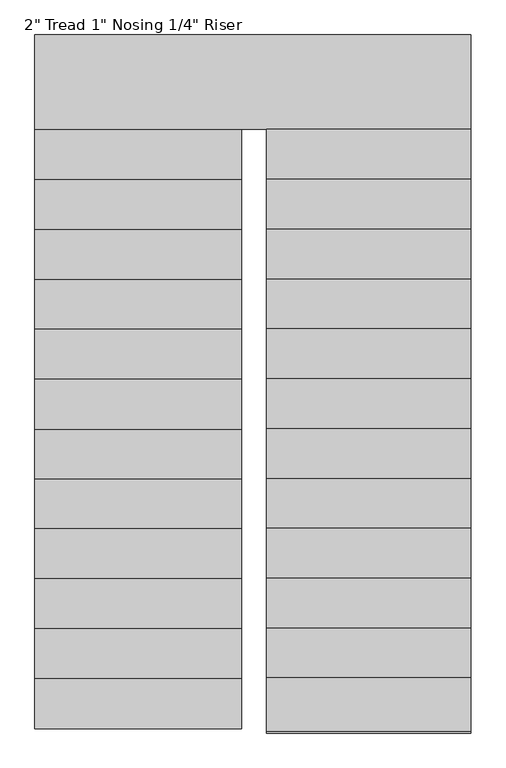
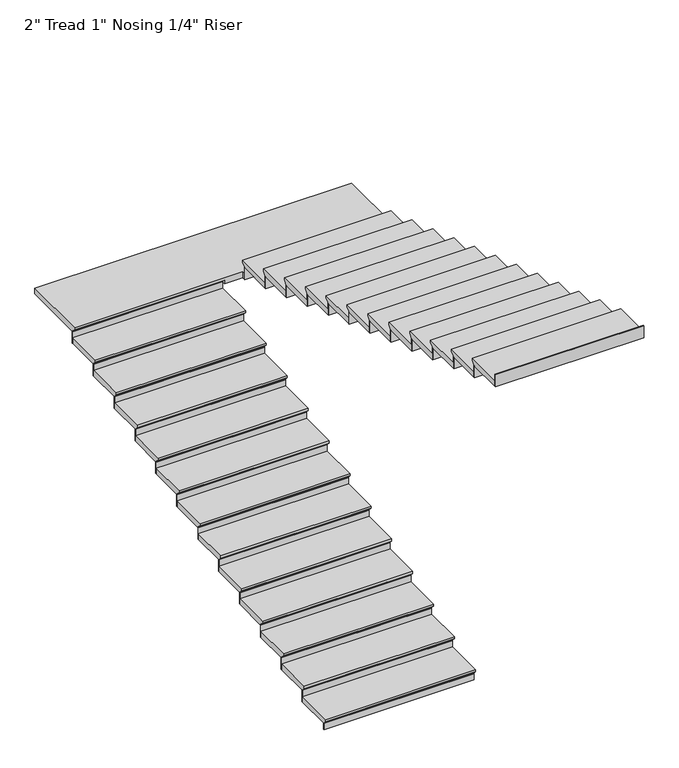
"""IFC4 building model written with IfcOpenShell, lengths in millimetres: stair flight geometry."""

from ifc_helpers import new_model, si_unit, origin, place, context, project, spatial, faceted_brep, source, transform, mapped, element, save


def stair_flight_6e2526ab(model_context):
    return source(origin(), model_context, "Body", "Brep", [
        faceted_brep([(-2593.7381751, -9955.5916506, 86.4576923), (-2593.7381751, -9955.5916506, 105.5076923), (-3857.687215, -9955.5916506, 105.5076923), (-3857.687215, -9955.5916506, 86.4576923), (-2593.7381751, -9930.1916506, 61.0576923), (-3857.687215, -9930.1916506, 61.0576923), (-2593.7381751, -9619.0416506, 105.5076923), (-3857.687215, -9619.0416506, 105.5076923), (-3857.687215, -9930.1916506, 54.7076923), (-3857.687215, -9619.0416506, 54.7076923), (-2593.7381751, -9619.0416506, 54.7076923), (-2593.7381751, -9930.1916506, 54.7076923)], [[[0, 1, 2, 3]], [[4, 0, 3, 5]], [[2, 1, 6, 7]], [[8, 9, 10, 11]], [[2, 7, 9, 8, 5, 3]], [[8, 11, 4, 5]], [[6, 1, 0, 4, 11, 10]], [[7, 6, 10, 9]]]),
        faceted_brep([(-2593.7381751, -9930.1916506, 54.7076923), (-2593.7381751, -9930.1916506, 0.0), (-2593.7381751, -9923.8416506, 0.0), (-2593.7381751, -9923.8416506, 54.7076923), (-3857.687215, -9930.1916506, 54.7076923), (-3857.687215, -9923.8416506, 54.7076923), (-3857.687215, -9923.8416506, 0.0), (-3857.687215, -9930.1916506, 0.0)], [[[0, 1, 2, 3]], [[4, 5, 6, 7]], [[1, 0, 4, 7]], [[2, 1, 7, 6]], [[3, 2, 6, 5]], [[0, 3, 5, 4]]]),
        faceted_brep([(-2593.7381751, -9619.0416506, 160.2153846), (-2593.7381751, -9619.0416506, 54.7076923), (-2593.7381751, -9612.6916506, 54.7076923), (-2593.7381751, -9612.6916506, 160.2153846), (-3857.687215, -9619.0416506, 160.2153846), (-3857.687215, -9612.6916506, 160.2153846), (-3857.687215, -9612.6916506, 54.7076923), (-3857.687215, -9619.0416506, 54.7076923)], [[[0, 1, 2, 3]], [[4, 5, 6, 7]], [[1, 0, 4, 7]], [[2, 1, 7, 6]], [[3, 2, 6, 5]], [[0, 3, 5, 4]]]),
        faceted_brep([(-3857.687215, -9644.4416506, 211.0153846), (-2593.7381751, -9644.4416506, 211.0153846), (-2593.7381751, -9314.2416506, 211.0153846), (-3857.687215, -9314.2416506, 211.0153846), (-3857.687215, -9619.0416506, 160.2153846), (-3857.687215, -9314.2416506, 160.2153846), (-2593.7381751, -9314.2416506, 160.2153846), (-2593.7381751, -9619.0416506, 160.2153846), (-3857.687215, -9619.0416506, 166.5653846), (-3857.687215, -9644.4416506, 191.9653846), (-2593.7381751, -9619.0416506, 166.5653846), (-2593.7381751, -9644.4416506, 191.9653846)], [[[0, 1, 2, 3]], [[4, 5, 6, 7]], [[0, 3, 5, 4, 8, 9]], [[4, 7, 10, 8]], [[2, 1, 11, 10, 7, 6]], [[3, 2, 6, 5]], [[11, 1, 0, 9]], [[10, 11, 9, 8]]]),
        faceted_brep([(-2593.7381751, -9314.2416506, 265.7230769), (-2593.7381751, -9314.2416506, 160.2153846), (-2593.7381751, -9307.8916506, 160.2153846), (-2593.7381751, -9307.8916506, 265.7230769), (-3857.687215, -9314.2416506, 265.7230769), (-3857.687215, -9307.8916506, 265.7230769), (-3857.687215, -9307.8916506, 160.2153846), (-3857.687215, -9314.2416506, 160.2153846)], [[[0, 1, 2, 3]], [[4, 5, 6, 7]], [[1, 0, 4, 7]], [[2, 1, 7, 6]], [[3, 2, 6, 5]], [[0, 3, 5, 4]]]),
        faceted_brep([(-3857.687215, -9339.6416506, 316.5230769), (-2593.7381751, -9339.6416506, 316.5230769), (-2593.7381751, -9009.4416506, 316.5230769), (-3857.687215, -9009.4416506, 316.5230769), (-3857.687215, -9314.2416506, 265.7230769), (-3857.687215, -9009.4416506, 265.7230769), (-2593.7381751, -9009.4416506, 265.7230769), (-2593.7381751, -9314.2416506, 265.7230769), (-3857.687215, -9314.2416506, 272.0730769), (-3857.687215, -9339.6416506, 297.4730769), (-2593.7381751, -9314.2416506, 272.0730769), (-2593.7381751, -9339.6416506, 297.4730769)], [[[0, 1, 2, 3]], [[4, 5, 6, 7]], [[0, 3, 5, 4, 8, 9]], [[4, 7, 10, 8]], [[2, 1, 11, 10, 7, 6]], [[3, 2, 6, 5]], [[11, 1, 0, 9]], [[10, 11, 9, 8]]]),
        faceted_brep([(-2593.7381751, -9009.4416506, 371.2307692), (-2593.7381751, -9009.4416506, 265.7230769), (-2593.7381751, -9003.0916506, 265.7230769), (-2593.7381751, -9003.0916506, 371.2307692), (-3857.687215, -9009.4416506, 371.2307692), (-3857.687215, -9003.0916506, 371.2307692), (-3857.687215, -9003.0916506, 265.7230769), (-3857.687215, -9009.4416506, 265.7230769)], [[[0, 1, 2, 3]], [[4, 5, 6, 7]], [[1, 0, 4, 7]], [[2, 1, 7, 6]], [[3, 2, 6, 5]], [[0, 3, 5, 4]]]),
        faceted_brep([(-3857.687215, -9034.8416506, 422.0307692), (-2593.7381751, -9034.8416506, 422.0307692), (-2593.7381751, -8704.6416506, 422.0307692), (-3857.687215, -8704.6416506, 422.0307692), (-3857.687215, -9009.4416506, 371.2307692), (-3857.687215, -8704.6416506, 371.2307692), (-2593.7381751, -8704.6416506, 371.2307692), (-2593.7381751, -9009.4416506, 371.2307692), (-3857.687215, -9009.4416506, 377.5807692), (-3857.687215, -9034.8416506, 402.9807692), (-2593.7381751, -9009.4416506, 377.5807692), (-2593.7381751, -9034.8416506, 402.9807692)], [[[0, 1, 2, 3]], [[4, 5, 6, 7]], [[0, 3, 5, 4, 8, 9]], [[4, 7, 10, 8]], [[2, 1, 11, 10, 7, 6]], [[3, 2, 6, 5]], [[11, 1, 0, 9]], [[10, 11, 9, 8]]]),
        faceted_brep([(-2593.7381751, -8704.6416506, 476.7384615), (-2593.7381751, -8704.6416506, 371.2307692), (-2593.7381751, -8698.2916506, 371.2307692), (-2593.7381751, -8698.2916506, 476.7384615), (-3857.687215, -8704.6416506, 476.7384615), (-3857.687215, -8698.2916506, 476.7384615), (-3857.687215, -8698.2916506, 371.2307692), (-3857.687215, -8704.6416506, 371.2307692)], [[[0, 1, 2, 3]], [[4, 5, 6, 7]], [[1, 0, 4, 7]], [[2, 1, 7, 6]], [[3, 2, 6, 5]], [[0, 3, 5, 4]]]),
        faceted_brep([(-3857.687215, -8730.0416506, 527.5384615), (-2593.7381751, -8730.0416506, 527.5384615), (-2593.7381751, -8399.8416506, 527.5384615), (-3857.687215, -8399.8416506, 527.5384615), (-3857.687215, -8704.6416506, 476.7384615), (-3857.687215, -8399.8416506, 476.7384615), (-2593.7381751, -8399.8416506, 476.7384615), (-2593.7381751, -8704.6416506, 476.7384615), (-3857.687215, -8704.6416506, 483.0884615), (-3857.687215, -8730.0416506, 508.4884615), (-2593.7381751, -8704.6416506, 483.0884615), (-2593.7381751, -8730.0416506, 508.4884615)], [[[0, 1, 2, 3]], [[4, 5, 6, 7]], [[0, 3, 5, 4, 8, 9]], [[4, 7, 10, 8]], [[2, 1, 11, 10, 7, 6]], [[3, 2, 6, 5]], [[11, 1, 0, 9]], [[10, 11, 9, 8]]]),
        faceted_brep([(-2593.7381751, -8399.8416506, 582.2461538), (-2593.7381751, -8399.8416506, 476.7384615), (-2593.7381751, -8393.4916506, 476.7384615), (-2593.7381751, -8393.4916506, 582.2461538), (-3857.687215, -8399.8416506, 582.2461538), (-3857.687215, -8393.4916506, 582.2461538), (-3857.687215, -8393.4916506, 476.7384615), (-3857.687215, -8399.8416506, 476.7384615)], [[[0, 1, 2, 3]], [[4, 5, 6, 7]], [[1, 0, 4, 7]], [[2, 1, 7, 6]], [[3, 2, 6, 5]], [[0, 3, 5, 4]]]),
        faceted_brep([(-3857.687215, -8425.2416506, 633.0461538), (-2593.7381751, -8425.2416506, 633.0461538), (-2593.7381751, -8098.2166506, 633.0461538), (-3857.687215, -8098.2166506, 633.0461538), (-3857.687215, -8399.8416506, 582.2461538), (-3857.687215, -8098.2166506, 582.2461538), (-2593.7381751, -8098.2166506, 582.2461538), (-2593.7381751, -8399.8416506, 582.2461538), (-3857.687215, -8399.8416506, 588.5961538), (-3857.687215, -8425.2416506, 613.9961538), (-2593.7381751, -8399.8416506, 588.5961538), (-2593.7381751, -8425.2416506, 613.9961538)], [[[0, 1, 2, 3]], [[4, 5, 6, 7]], [[0, 3, 5, 4, 8, 9]], [[4, 7, 10, 8]], [[2, 1, 11, 10, 7, 6]], [[3, 2, 6, 5]], [[11, 1, 0, 9]], [[10, 11, 9, 8]]]),
        faceted_brep([(-2593.7381751, -8098.2166506, 687.7538462), (-2593.7381751, -8098.2166506, 582.2461538), (-2593.7381751, -8091.8666506, 582.2461538), (-2593.7381751, -8091.8666506, 687.7538462), (-3857.687215, -8098.2166506, 687.7538462), (-3857.687215, -8091.8666506, 687.7538462), (-3857.687215, -8091.8666506, 582.2461538), (-3857.687215, -8098.2166506, 582.2461538)], [[[0, 1, 2, 3]], [[4, 5, 6, 7]], [[1, 0, 4, 7]], [[2, 1, 7, 6]], [[3, 2, 6, 5]], [[0, 3, 5, 4]]]),
        faceted_brep([(-3857.687215, -8123.6166506, 738.5538462), (-2593.7381751, -8123.6166506, 738.5538462), (-2593.7381751, -7790.2416506, 738.5538462), (-3857.687215, -7790.2416506, 738.5538462), (-3857.687215, -8098.2166506, 687.7538462), (-3857.687215, -7790.2416506, 687.7538462), (-2593.7381751, -7790.2416506, 687.7538462), (-2593.7381751, -8098.2166506, 687.7538462), (-3857.687215, -8098.2166506, 694.1038462), (-3857.687215, -8123.6166506, 719.5038462), (-2593.7381751, -8098.2166506, 694.1038462), (-2593.7381751, -8123.6166506, 719.5038462)], [[[0, 1, 2, 3]], [[4, 5, 6, 7]], [[0, 3, 5, 4, 8, 9]], [[4, 7, 10, 8]], [[2, 1, 11, 10, 7, 6]], [[3, 2, 6, 5]], [[11, 1, 0, 9]], [[10, 11, 9, 8]]]),
        faceted_brep([(-2593.7381751, -7790.2416506, 793.2615385), (-2593.7381751, -7790.2416506, 687.7538462), (-2593.7381751, -7783.8916506, 687.7538462), (-2593.7381751, -7783.8916506, 793.2615385), (-3857.687215, -7790.2416506, 793.2615385), (-3857.687215, -7783.8916506, 793.2615385), (-3857.687215, -7783.8916506, 687.7538462), (-3857.687215, -7790.2416506, 687.7538462)], [[[0, 1, 2, 3]], [[4, 5, 6, 7]], [[1, 0, 4, 7]], [[2, 1, 7, 6]], [[3, 2, 6, 5]], [[0, 3, 5, 4]]]),
        faceted_brep([(-3857.687215, -7815.6416506, 844.0615385), (-2593.7381751, -7815.6416506, 844.0615385), (-2593.7381751, -7485.4416506, 844.0615385), (-3857.687215, -7485.4416506, 844.0615385), (-3857.687215, -7790.2416506, 793.2615385), (-3857.687215, -7485.4416506, 793.2615385), (-2593.7381751, -7485.4416506, 793.2615385), (-2593.7381751, -7790.2416506, 793.2615385), (-3857.687215, -7790.2416506, 799.6115385), (-3857.687215, -7815.6416506, 825.0115385), (-2593.7381751, -7790.2416506, 799.6115385), (-2593.7381751, -7815.6416506, 825.0115385)], [[[0, 1, 2, 3]], [[4, 5, 6, 7]], [[0, 3, 5, 4, 8, 9]], [[4, 7, 10, 8]], [[2, 1, 11, 10, 7, 6]], [[3, 2, 6, 5]], [[11, 1, 0, 9]], [[10, 11, 9, 8]]]),
        faceted_brep([(-2593.7381751, -7485.4416506, 898.7692308), (-2593.7381751, -7485.4416506, 793.2615385), (-2593.7381751, -7479.0916506, 793.2615385), (-2593.7381751, -7479.0916506, 898.7692308), (-3857.687215, -7485.4416506, 898.7692308), (-3857.687215, -7479.0916506, 898.7692308), (-3857.687215, -7479.0916506, 793.2615385), (-3857.687215, -7485.4416506, 793.2615385)], [[[0, 1, 2, 3]], [[4, 5, 6, 7]], [[1, 0, 4, 7]], [[2, 1, 7, 6]], [[3, 2, 6, 5]], [[0, 3, 5, 4]]]),
        faceted_brep([(-3857.687215, -7510.8416506, 949.5692308), (-2593.7381751, -7510.8416506, 949.5692308), (-2593.7381751, -7180.6416506, 949.5692308), (-3857.687215, -7180.6416506, 949.5692308), (-3857.687215, -7485.4416506, 898.7692308), (-3857.687215, -7180.6416506, 898.7692308), (-2593.7381751, -7180.6416506, 898.7692308), (-2593.7381751, -7485.4416506, 898.7692308), (-3857.687215, -7485.4416506, 905.1192308), (-3857.687215, -7510.8416506, 930.5192308), (-2593.7381751, -7485.4416506, 905.1192308), (-2593.7381751, -7510.8416506, 930.5192308)], [[[0, 1, 2, 3]], [[4, 5, 6, 7]], [[0, 3, 5, 4, 8, 9]], [[4, 7, 10, 8]], [[2, 1, 11, 10, 7, 6]], [[3, 2, 6, 5]], [[11, 1, 0, 9]], [[10, 11, 9, 8]]]),
        faceted_brep([(-2593.7381751, -7180.6416506, 1004.2769231), (-2593.7381751, -7180.6416506, 898.7692308), (-2593.7381751, -7174.2916506, 898.7692308), (-2593.7381751, -7174.2916506, 1004.2769231), (-3857.687215, -7180.6416506, 1004.2769231), (-3857.687215, -7174.2916506, 1004.2769231), (-3857.687215, -7174.2916506, 898.7692308), (-3857.687215, -7180.6416506, 898.7692308)], [[[0, 1, 2, 3]], [[4, 5, 6, 7]], [[1, 0, 4, 7]], [[2, 1, 7, 6]], [[3, 2, 6, 5]], [[0, 3, 5, 4]]]),
        faceted_brep([(-3857.687215, -7206.0416506, 1055.0769231), (-2593.7381751, -7206.0416506, 1055.0769231), (-2593.7381751, -6875.8416506, 1055.0769231), (-3857.687215, -6875.8416506, 1055.0769231), (-3857.687215, -7180.6416506, 1004.2769231), (-3857.687215, -6875.8416506, 1004.2769231), (-2593.7381751, -6875.8416506, 1004.2769231), (-2593.7381751, -7180.6416506, 1004.2769231), (-3857.687215, -7180.6416506, 1010.6269231), (-3857.687215, -7206.0416506, 1036.0269231), (-2593.7381751, -7180.6416506, 1010.6269231), (-2593.7381751, -7206.0416506, 1036.0269231)], [[[0, 1, 2, 3]], [[4, 5, 6, 7]], [[0, 3, 5, 4, 8, 9]], [[4, 7, 10, 8]], [[2, 1, 11, 10, 7, 6]], [[3, 2, 6, 5]], [[11, 1, 0, 9]], [[10, 11, 9, 8]]]),
        faceted_brep([(-2593.7381751, -6875.8416506, 1109.7846154), (-2593.7381751, -6875.8416506, 1004.2769231), (-2593.7381751, -6869.4916506, 1004.2769231), (-2593.7381751, -6869.4916506, 1109.7846154), (-3857.687215, -6875.8416506, 1109.7846154), (-3857.687215, -6869.4916506, 1109.7846154), (-3857.687215, -6869.4916506, 1004.2769231), (-3857.687215, -6875.8416506, 1004.2769231)], [[[0, 1, 2, 3]], [[4, 5, 6, 7]], [[1, 0, 4, 7]], [[2, 1, 7, 6]], [[3, 2, 6, 5]], [[0, 3, 5, 4]]]),
        faceted_brep([(-3857.687215, -6901.2416506, 1160.5846154), (-2593.7381751, -6901.2416506, 1160.5846154), (-2593.7381751, -6571.0416506, 1160.5846154), (-3857.687215, -6571.0416506, 1160.5846154), (-3857.687215, -6875.8416506, 1109.7846154), (-3857.687215, -6571.0416506, 1109.7846154), (-2593.7381751, -6571.0416506, 1109.7846154), (-2593.7381751, -6875.8416506, 1109.7846154), (-3857.687215, -6875.8416506, 1116.1346154), (-3857.687215, -6901.2416506, 1141.5346154), (-2593.7381751, -6875.8416506, 1116.1346154), (-2593.7381751, -6901.2416506, 1141.5346154)], [[[0, 1, 2, 3]], [[4, 5, 6, 7]], [[0, 3, 5, 4, 8, 9]], [[4, 7, 10, 8]], [[2, 1, 11, 10, 7, 6]], [[3, 2, 6, 5]], [[11, 1, 0, 9]], [[10, 11, 9, 8]]]),
        faceted_brep([(-2593.7381751, -6571.0416506, 1215.2923077), (-2593.7381751, -6571.0416506, 1109.7846154), (-2593.7381751, -6564.6916506, 1109.7846154), (-2593.7381751, -6564.6916506, 1215.2923077), (-3857.687215, -6571.0416506, 1215.2923077), (-3857.687215, -6564.6916506, 1215.2923077), (-3857.687215, -6564.6916506, 1109.7846154), (-3857.687215, -6571.0416506, 1109.7846154)], [[[0, 1, 2, 3]], [[4, 5, 6, 7]], [[1, 0, 4, 7]], [[2, 1, 7, 6]], [[3, 2, 6, 5]], [[0, 3, 5, 4]]]),
        faceted_brep([(-3857.687215, -6596.4416506, 1266.0923077), (-2593.7381751, -6596.4416506, 1266.0923077), (-2593.7381751, -6266.2416506, 1266.0923077), (-3857.687215, -6266.2416506, 1266.0923077), (-3857.687215, -6571.0416506, 1215.2923077), (-3857.687215, -6266.2416506, 1215.2923077), (-2593.7381751, -6266.2416506, 1215.2923077), (-2593.7381751, -6571.0416506, 1215.2923077), (-3857.687215, -6571.0416506, 1221.6423077), (-3857.687215, -6596.4416506, 1247.0423077), (-2593.7381751, -6571.0416506, 1221.6423077), (-2593.7381751, -6596.4416506, 1247.0423077)], [[[0, 1, 2, 3]], [[4, 5, 6, 7]], [[0, 3, 5, 4, 8, 9]], [[4, 7, 10, 8]], [[2, 1, 11, 10, 7, 6]], [[3, 2, 6, 5]], [[11, 1, 0, 9]], [[10, 11, 9, 8]]]),
        faceted_brep([(-2593.7381751, -6266.2416506, 1320.8), (-2593.7381751, -6266.2416506, 1215.2923077), (-2593.7381751, -6259.8916506, 1215.2923077), (-2593.7381751, -6259.8916506, 1320.8), (-3857.687215, -6266.2416506, 1320.8), (-3857.687215, -6259.8916506, 1320.8), (-3857.687215, -6259.8916506, 1215.2923077), (-3857.687215, -6266.2416506, 1215.2923077)], [[[0, 1, 2, 3]], [[4, 5, 6, 7]], [[1, 0, 4, 7]], [[2, 1, 7, 6]], [[3, 2, 6, 5]], [[0, 3, 5, 4]]]),
        faceted_brep([(-1190.687215, -6317.0416506, 1371.6), (-1190.687215, -5713.7916506, 1371.6), (-3857.687215, -5713.7916506, 1371.6), (-3857.687215, -6291.6416506, 1371.6), (-2441.3381751, -6291.6416506, 1371.6), (-2441.3381751, -6317.0416506, 1371.6), (-1190.687215, -5713.7916506, 1320.8), (-1190.687215, -6317.0416506, 1320.8), (-2441.3381751, -6317.0416506, 1320.8), (-2441.3381751, -6291.6416506, 1320.8), (-2593.7381751, -6291.6416506, 1320.8), (-2593.7381751, -6266.2416506, 1320.8), (-3857.687215, -6266.2416506, 1320.8), (-3857.687215, -5713.7916506, 1320.8), (-3857.687215, -6266.2416506, 1327.15), (-3857.687215, -6291.6416506, 1352.55), (-2593.7381751, -6266.2416506, 1327.15), (-2593.7381751, -6291.6416506, 1352.55)], [[[0, 1, 2, 3, 4, 5]], [[6, 7, 8, 9, 10, 11, 12, 13]], [[1, 0, 7, 6]], [[2, 1, 6, 13]], [[3, 2, 13, 12, 14, 15]], [[12, 11, 16, 14]], [[11, 10, 17, 16]], [[4, 3, 15, 17, 10, 9]], [[5, 4, 9, 8]], [[0, 5, 8, 7]], [[15, 14, 16, 17]]]),
        faceted_brep([(-2441.3381751, -6317.0416506, 1426.3076923), (-2441.3381751, -6317.0416506, 1320.8), (-2441.3381751, -6323.3916506, 1320.8), (-2441.3381751, -6323.3916506, 1426.3076923), (-1190.687215, -6317.0416506, 1426.3076923), (-1190.687215, -6323.3916506, 1426.3076923), (-1190.687215, -6323.3916506, 1320.8), (-1190.687215, -6317.0416506, 1320.8)], [[[0, 1, 2, 3]], [[4, 5, 6, 7]], [[1, 0, 4, 7]], [[2, 1, 7, 6]], [[3, 2, 6, 5]], [[0, 3, 5, 4]]]),
        faceted_brep([(-1190.687215, -6291.6416506, 1477.1076923), (-2441.3381751, -6291.6416506, 1477.1076923), (-2441.3381751, -6621.8416506, 1477.1076923), (-1190.687215, -6621.8416506, 1477.1076923), (-1190.687215, -6317.0416506, 1426.3076923), (-1190.687215, -6621.8416506, 1426.3076923), (-2441.3381751, -6621.8416506, 1426.3076923), (-2441.3381751, -6317.0416506, 1426.3076923), (-1190.687215, -6317.0416506, 1432.6576923), (-1190.687215, -6291.6416506, 1458.0576923), (-2441.3381751, -6317.0416506, 1432.6576923), (-2441.3381751, -6291.6416506, 1458.0576923)], [[[0, 1, 2, 3]], [[4, 5, 6, 7]], [[0, 3, 5, 4, 8, 9]], [[4, 7, 10, 8]], [[2, 1, 11, 10, 7, 6]], [[3, 2, 6, 5]], [[11, 1, 0, 9]], [[10, 11, 9, 8]]]),
        faceted_brep([(-2441.3381751, -6621.8416506, 1531.8153846), (-2441.3381751, -6621.8416506, 1426.3076923), (-2441.3381751, -6628.1916506, 1426.3076923), (-2441.3381751, -6628.1916506, 1531.8153846), (-1190.687215, -6621.8416506, 1531.8153846), (-1190.687215, -6628.1916506, 1531.8153846), (-1190.687215, -6628.1916506, 1426.3076923), (-1190.687215, -6621.8416506, 1426.3076923)], [[[0, 1, 2, 3]], [[4, 5, 6, 7]], [[1, 0, 4, 7]], [[2, 1, 7, 6]], [[3, 2, 6, 5]], [[0, 3, 5, 4]]]),
        faceted_brep([(-1190.687215, -6596.4416506, 1582.6153846), (-2441.3381751, -6596.4416506, 1582.6153846), (-2441.3381751, -6926.6416506, 1582.6153846), (-1190.687215, -6926.6416506, 1582.6153846), (-1190.687215, -6621.8416506, 1531.8153846), (-1190.687215, -6926.6416506, 1531.8153846), (-2441.3381751, -6926.6416506, 1531.8153846), (-2441.3381751, -6621.8416506, 1531.8153846), (-1190.687215, -6621.8416506, 1538.1653846), (-1190.687215, -6596.4416506, 1563.5653846), (-2441.3381751, -6621.8416506, 1538.1653846), (-2441.3381751, -6596.4416506, 1563.5653846)], [[[0, 1, 2, 3]], [[4, 5, 6, 7]], [[0, 3, 5, 4, 8, 9]], [[4, 7, 10, 8]], [[2, 1, 11, 10, 7, 6]], [[3, 2, 6, 5]], [[11, 1, 0, 9]], [[10, 11, 9, 8]]]),
        faceted_brep([(-2441.3381751, -6926.6416506, 1637.3230769), (-2441.3381751, -6926.6416506, 1531.8153846), (-2441.3381751, -6932.9916506, 1531.8153846), (-2441.3381751, -6932.9916506, 1637.3230769), (-1190.687215, -6926.6416506, 1637.3230769), (-1190.687215, -6932.9916506, 1637.3230769), (-1190.687215, -6932.9916506, 1531.8153846), (-1190.687215, -6926.6416506, 1531.8153846)], [[[0, 1, 2, 3]], [[4, 5, 6, 7]], [[1, 0, 4, 7]], [[2, 1, 7, 6]], [[3, 2, 6, 5]], [[0, 3, 5, 4]]]),
        faceted_brep([(-1190.687215, -6901.2416506, 1688.1230769), (-2441.3381751, -6901.2416506, 1688.1230769), (-2441.3381751, -7231.4416506, 1688.1230769), (-1190.687215, -7231.4416506, 1688.1230769), (-1190.687215, -6926.6416506, 1637.3230769), (-1190.687215, -7231.4416506, 1637.3230769), (-2441.3381751, -7231.4416506, 1637.3230769), (-2441.3381751, -6926.6416506, 1637.3230769), (-1190.687215, -6926.6416506, 1643.6730769), (-1190.687215, -6901.2416506, 1669.0730769), (-2441.3381751, -6926.6416506, 1643.6730769), (-2441.3381751, -6901.2416506, 1669.0730769)], [[[0, 1, 2, 3]], [[4, 5, 6, 7]], [[0, 3, 5, 4, 8, 9]], [[4, 7, 10, 8]], [[2, 1, 11, 10, 7, 6]], [[3, 2, 6, 5]], [[11, 1, 0, 9]], [[10, 11, 9, 8]]]),
        faceted_brep([(-2441.3381751, -7231.4416506, 1742.8307692), (-2441.3381751, -7231.4416506, 1637.3230769), (-2441.3381751, -7237.7916506, 1637.3230769), (-2441.3381751, -7237.7916506, 1742.8307692), (-1190.687215, -7231.4416506, 1742.8307692), (-1190.687215, -7237.7916506, 1742.8307692), (-1190.687215, -7237.7916506, 1637.3230769), (-1190.687215, -7231.4416506, 1637.3230769)], [[[0, 1, 2, 3]], [[4, 5, 6, 7]], [[1, 0, 4, 7]], [[2, 1, 7, 6]], [[3, 2, 6, 5]], [[0, 3, 5, 4]]]),
        faceted_brep([(-1190.687215, -7206.0416506, 1793.6307692), (-2441.3381751, -7206.0416506, 1793.6307692), (-2441.3381751, -7536.2416506, 1793.6307692), (-1190.687215, -7536.2416506, 1793.6307692), (-1190.687215, -7231.4416506, 1742.8307692), (-1190.687215, -7536.2416506, 1742.8307692), (-2441.3381751, -7536.2416506, 1742.8307692), (-2441.3381751, -7231.4416506, 1742.8307692), (-1190.687215, -7231.4416506, 1749.1807692), (-1190.687215, -7206.0416506, 1774.5807692), (-2441.3381751, -7231.4416506, 1749.1807692), (-2441.3381751, -7206.0416506, 1774.5807692)], [[[0, 1, 2, 3]], [[4, 5, 6, 7]], [[0, 3, 5, 4, 8, 9]], [[4, 7, 10, 8]], [[2, 1, 11, 10, 7, 6]], [[3, 2, 6, 5]], [[11, 1, 0, 9]], [[10, 11, 9, 8]]]),
        faceted_brep([(-2441.3381751, -7536.2416506, 1848.3384615), (-2441.3381751, -7536.2416506, 1742.8307692), (-2441.3381751, -7542.5916506, 1742.8307692), (-2441.3381751, -7542.5916506, 1848.3384615), (-1190.687215, -7536.2416506, 1848.3384615), (-1190.687215, -7542.5916506, 1848.3384615), (-1190.687215, -7542.5916506, 1742.8307692), (-1190.687215, -7536.2416506, 1742.8307692)], [[[0, 1, 2, 3]], [[4, 5, 6, 7]], [[1, 0, 4, 7]], [[2, 1, 7, 6]], [[3, 2, 6, 5]], [[0, 3, 5, 4]]]),
        faceted_brep([(-1190.687215, -7510.8416506, 1899.1384615), (-2441.3381751, -7510.8416506, 1899.1384615), (-2441.3381751, -7841.0416506, 1899.1384615), (-1190.687215, -7841.0416506, 1899.1384615), (-1190.687215, -7536.2416506, 1848.3384615), (-1190.687215, -7841.0416506, 1848.3384615), (-2441.3381751, -7841.0416506, 1848.3384615), (-2441.3381751, -7536.2416506, 1848.3384615), (-1190.687215, -7536.2416506, 1854.6884615), (-1190.687215, -7510.8416506, 1880.0884615), (-2441.3381751, -7536.2416506, 1854.6884615), (-2441.3381751, -7510.8416506, 1880.0884615)], [[[0, 1, 2, 3]], [[4, 5, 6, 7]], [[0, 3, 5, 4, 8, 9]], [[4, 7, 10, 8]], [[2, 1, 11, 10, 7, 6]], [[3, 2, 6, 5]], [[11, 1, 0, 9]], [[10, 11, 9, 8]]]),
        faceted_brep([(-2441.3381751, -7841.0416506, 1953.8461538), (-2441.3381751, -7841.0416506, 1848.3384615), (-2441.3381751, -7847.3916506, 1848.3384615), (-2441.3381751, -7847.3916506, 1953.8461538), (-1190.687215, -7841.0416506, 1953.8461538), (-1190.687215, -7847.3916506, 1953.8461538), (-1190.687215, -7847.3916506, 1848.3384615), (-1190.687215, -7841.0416506, 1848.3384615)], [[[0, 1, 2, 3]], [[4, 5, 6, 7]], [[1, 0, 4, 7]], [[2, 1, 7, 6]], [[3, 2, 6, 5]], [[0, 3, 5, 4]]]),
        faceted_brep([(-1190.687215, -7815.6416506, 2004.6461538), (-2441.3381751, -7815.6416506, 2004.6461538), (-2441.3381751, -8145.8416506, 2004.6461538), (-1190.687215, -8145.8416506, 2004.6461538), (-1190.687215, -7841.0416506, 1953.8461538), (-1190.687215, -8145.8416506, 1953.8461538), (-2441.3381751, -8145.8416506, 1953.8461538), (-2441.3381751, -7841.0416506, 1953.8461538), (-1190.687215, -7841.0416506, 1960.1961538), (-1190.687215, -7815.6416506, 1985.5961538), (-2441.3381751, -7841.0416506, 1960.1961538), (-2441.3381751, -7815.6416506, 1985.5961538)], [[[0, 1, 2, 3]], [[4, 5, 6, 7]], [[0, 3, 5, 4, 8, 9]], [[4, 7, 10, 8]], [[2, 1, 11, 10, 7, 6]], [[3, 2, 6, 5]], [[11, 1, 0, 9]], [[10, 11, 9, 8]]]),
        faceted_brep([(-2441.3381751, -8145.8416506, 2059.3538462), (-2441.3381751, -8145.8416506, 1953.8461538), (-2441.3381751, -8152.1916506, 1953.8461538), (-2441.3381751, -8152.1916506, 2059.3538462), (-1190.687215, -8145.8416506, 2059.3538462), (-1190.687215, -8152.1916506, 2059.3538462), (-1190.687215, -8152.1916506, 1953.8461538), (-1190.687215, -8145.8416506, 1953.8461538)], [[[0, 1, 2, 3]], [[4, 5, 6, 7]], [[1, 0, 4, 7]], [[2, 1, 7, 6]], [[3, 2, 6, 5]], [[0, 3, 5, 4]]]),
        faceted_brep([(-1190.687215, -8120.4416506, 2110.1538462), (-2441.3381751, -8120.4416506, 2110.1538462), (-2441.3381751, -8450.6416506, 2110.1538462), (-1190.687215, -8450.6416506, 2110.1538462), (-1190.687215, -8145.8416506, 2059.3538462), (-1190.687215, -8450.6416506, 2059.3538462), (-2441.3381751, -8450.6416506, 2059.3538462), (-2441.3381751, -8145.8416506, 2059.3538462), (-1190.687215, -8145.8416506, 2065.7038462), (-1190.687215, -8120.4416506, 2091.1038462), (-2441.3381751, -8145.8416506, 2065.7038462), (-2441.3381751, -8120.4416506, 2091.1038462)], [[[0, 1, 2, 3]], [[4, 5, 6, 7]], [[0, 3, 5, 4, 8, 9]], [[4, 7, 10, 8]], [[2, 1, 11, 10, 7, 6]], [[3, 2, 6, 5]], [[11, 1, 0, 9]], [[10, 11, 9, 8]]]),
        faceted_brep([(-2441.3381751, -8450.6416506, 2164.8615385), (-2441.3381751, -8450.6416506, 2059.3538462), (-2441.3381751, -8456.9916506, 2059.3538462), (-2441.3381751, -8456.9916506, 2164.8615385), (-1190.687215, -8450.6416506, 2164.8615385), (-1190.687215, -8456.9916506, 2164.8615385), (-1190.687215, -8456.9916506, 2059.3538462), (-1190.687215, -8450.6416506, 2059.3538462)], [[[0, 1, 2, 3]], [[4, 5, 6, 7]], [[1, 0, 4, 7]], [[2, 1, 7, 6]], [[3, 2, 6, 5]], [[0, 3, 5, 4]]]),
        faceted_brep([(-1190.687215, -8425.2416506, 2215.6615385), (-2441.3381751, -8425.2416506, 2215.6615385), (-2441.3381751, -8755.4416506, 2215.6615385), (-1190.687215, -8755.4416506, 2215.6615385), (-1190.687215, -8450.6416506, 2164.8615385), (-1190.687215, -8755.4416506, 2164.8615385), (-2441.3381751, -8755.4416506, 2164.8615385), (-2441.3381751, -8450.6416506, 2164.8615385), (-1190.687215, -8450.6416506, 2171.2115385), (-1190.687215, -8425.2416506, 2196.6115385), (-2441.3381751, -8450.6416506, 2171.2115385), (-2441.3381751, -8425.2416506, 2196.6115385)], [[[0, 1, 2, 3]], [[4, 5, 6, 7]], [[0, 3, 5, 4, 8, 9]], [[4, 7, 10, 8]], [[2, 1, 11, 10, 7, 6]], [[3, 2, 6, 5]], [[11, 1, 0, 9]], [[10, 11, 9, 8]]]),
        faceted_brep([(-2441.3381751, -8755.4416506, 2270.3692308), (-2441.3381751, -8755.4416506, 2164.8615385), (-2441.3381751, -8761.7916506, 2164.8615385), (-2441.3381751, -8761.7916506, 2270.3692308), (-1190.687215, -8755.4416506, 2270.3692308), (-1190.687215, -8761.7916506, 2270.3692308), (-1190.687215, -8761.7916506, 2164.8615385), (-1190.687215, -8755.4416506, 2164.8615385)], [[[0, 1, 2, 3]], [[4, 5, 6, 7]], [[1, 0, 4, 7]], [[2, 1, 7, 6]], [[3, 2, 6, 5]], [[0, 3, 5, 4]]]),
        faceted_brep([(-1190.687215, -8730.0416506, 2321.1692308), (-2441.3381751, -8730.0416506, 2321.1692308), (-2441.3381751, -9060.2416506, 2321.1692308), (-1190.687215, -9060.2416506, 2321.1692308), (-1190.687215, -8755.4416506, 2270.3692308), (-1190.687215, -9060.2416506, 2270.3692308), (-2441.3381751, -9060.2416506, 2270.3692308), (-2441.3381751, -8755.4416506, 2270.3692308), (-1190.687215, -8755.4416506, 2276.7192308), (-1190.687215, -8730.0416506, 2302.1192308), (-2441.3381751, -8755.4416506, 2276.7192308), (-2441.3381751, -8730.0416506, 2302.1192308)], [[[0, 1, 2, 3]], [[4, 5, 6, 7]], [[0, 3, 5, 4, 8, 9]], [[4, 7, 10, 8]], [[2, 1, 11, 10, 7, 6]], [[3, 2, 6, 5]], [[11, 1, 0, 9]], [[10, 11, 9, 8]]]),
        faceted_brep([(-2441.3381751, -9060.2416506, 2375.8769231), (-2441.3381751, -9060.2416506, 2270.3692308), (-2441.3381751, -9066.5916506, 2270.3692308), (-2441.3381751, -9066.5916506, 2375.8769231), (-1190.687215, -9060.2416506, 2375.8769231), (-1190.687215, -9066.5916506, 2375.8769231), (-1190.687215, -9066.5916506, 2270.3692308), (-1190.687215, -9060.2416506, 2270.3692308)], [[[0, 1, 2, 3]], [[4, 5, 6, 7]], [[1, 0, 4, 7]], [[2, 1, 7, 6]], [[3, 2, 6, 5]], [[0, 3, 5, 4]]]),
        faceted_brep([(-1190.687215, -9034.8416506, 2426.6769231), (-2441.3381751, -9034.8416506, 2426.6769231), (-2441.3381751, -9365.0416506, 2426.6769231), (-1190.687215, -9365.0416506, 2426.6769231), (-1190.687215, -9060.2416506, 2375.8769231), (-1190.687215, -9365.0416506, 2375.8769231), (-2441.3381751, -9365.0416506, 2375.8769231), (-2441.3381751, -9060.2416506, 2375.8769231), (-1190.687215, -9060.2416506, 2382.2269231), (-1190.687215, -9034.8416506, 2407.6269231), (-2441.3381751, -9060.2416506, 2382.2269231), (-2441.3381751, -9034.8416506, 2407.6269231)], [[[0, 1, 2, 3]], [[4, 5, 6, 7]], [[0, 3, 5, 4, 8, 9]], [[4, 7, 10, 8]], [[2, 1, 11, 10, 7, 6]], [[3, 2, 6, 5]], [[11, 1, 0, 9]], [[10, 11, 9, 8]]]),
        faceted_brep([(-2441.3381751, -9365.0416506, 2481.3846154), (-2441.3381751, -9365.0416506, 2375.8769231), (-2441.3381751, -9371.3916506, 2375.8769231), (-2441.3381751, -9371.3916506, 2481.3846154), (-1190.687215, -9365.0416506, 2481.3846154), (-1190.687215, -9371.3916506, 2481.3846154), (-1190.687215, -9371.3916506, 2375.8769231), (-1190.687215, -9365.0416506, 2375.8769231)], [[[0, 1, 2, 3]], [[4, 5, 6, 7]], [[1, 0, 4, 7]], [[2, 1, 7, 6]], [[3, 2, 6, 5]], [[0, 3, 5, 4]]]),
        faceted_brep([(-1190.687215, -9339.6416506, 2532.1846154), (-2441.3381751, -9339.6416506, 2532.1846154), (-2441.3381751, -9669.8416506, 2532.1846154), (-1190.687215, -9669.8416506, 2532.1846154), (-1190.687215, -9365.0416506, 2481.3846154), (-1190.687215, -9669.8416506, 2481.3846154), (-2441.3381751, -9669.8416506, 2481.3846154), (-2441.3381751, -9365.0416506, 2481.3846154), (-1190.687215, -9365.0416506, 2487.7346154), (-1190.687215, -9339.6416506, 2513.1346154), (-2441.3381751, -9365.0416506, 2487.7346154), (-2441.3381751, -9339.6416506, 2513.1346154)], [[[0, 1, 2, 3]], [[4, 5, 6, 7]], [[0, 3, 5, 4, 8, 9]], [[4, 7, 10, 8]], [[2, 1, 11, 10, 7, 6]], [[3, 2, 6, 5]], [[11, 1, 0, 9]], [[10, 11, 9, 8]]]),
        faceted_brep([(-2441.3381751, -9669.8416506, 2586.8923077), (-2441.3381751, -9669.8416506, 2481.3846154), (-2441.3381751, -9676.1916506, 2481.3846154), (-2441.3381751, -9676.1916506, 2586.8923077), (-1190.687215, -9669.8416506, 2586.8923077), (-1190.687215, -9676.1916506, 2586.8923077), (-1190.687215, -9676.1916506, 2481.3846154), (-1190.687215, -9669.8416506, 2481.3846154)], [[[0, 1, 2, 3]], [[4, 5, 6, 7]], [[1, 0, 4, 7]], [[2, 1, 7, 6]], [[3, 2, 6, 5]], [[0, 3, 5, 4]]]),
        faceted_brep([(-2441.3381751, -9974.6416506, 2692.4), (-2441.3381751, -9974.6416506, 2586.8923077), (-2441.3381751, -9980.9916506, 2586.8923077), (-2441.3381751, -9980.9916506, 2692.4), (-1190.687215, -9974.6416506, 2692.4), (-1190.687215, -9980.9916506, 2692.4), (-1190.687215, -9980.9916506, 2586.8923077), (-1190.687215, -9974.6416506, 2586.8923077)], [[[0, 1, 2, 3]], [[4, 5, 6, 7]], [[1, 0, 4, 7]], [[2, 1, 7, 6]], [[3, 2, 6, 5]], [[0, 3, 5, 4]]]),
        faceted_brep([(-1190.687215, -9644.4416506, 2637.6923077), (-2441.3381751, -9644.4416506, 2637.6923077), (-2441.3381751, -9974.6416506, 2637.6923077), (-1190.687215, -9974.6416506, 2637.6923077), (-1190.687215, -9669.8416506, 2586.8923077), (-1190.687215, -9974.6416506, 2586.8923077), (-2441.3381751, -9974.6416506, 2586.8923077), (-2441.3381751, -9669.8416506, 2586.8923077), (-1190.687215, -9669.8416506, 2593.2423077), (-1190.687215, -9644.4416506, 2618.6423077), (-2441.3381751, -9669.8416506, 2593.2423077), (-2441.3381751, -9644.4416506, 2618.6423077)], [[[0, 1, 2, 3]], [[4, 5, 6, 7]], [[0, 3, 5, 4, 8, 9]], [[4, 7, 10, 8]], [[2, 1, 11, 10, 7, 6]], [[3, 2, 6, 5]], [[11, 1, 0, 9]], [[10, 11, 9, 8]]]),
    ])


if __name__ == "__main__":
    model = new_model("IFC4")
    model_context = context("Model", 3, world=origin())
    ifc_project = project(units=[si_unit("LENGTHUNIT", "METRE", prefix="MILLI")], contexts=[model_context])
    site = spatial("IfcSite", under=ifc_project)
    building = spatial("IfcBuilding", under=site)
    placement = place(None, origin())
    stair_flight_shape = stair_flight_6e2526ab(model_context)
    element("IfcStairFlight", 1, ObjectType="2\" Tread 1\" Nosing 1/4\" Riser", at=placement, inside=building, context=model_context, shape_type="MappedRepresentation", body=[
        mapped(stair_flight_shape, transform((0.0, 0.0, 0.0), x_axis=(1.0, 0.0, 0.0), y_axis=(0.0, 1.0, 0.0), z_axis=(0.0, 0.0, 1.0))),
    ])
    save(model, "model.ifc")
